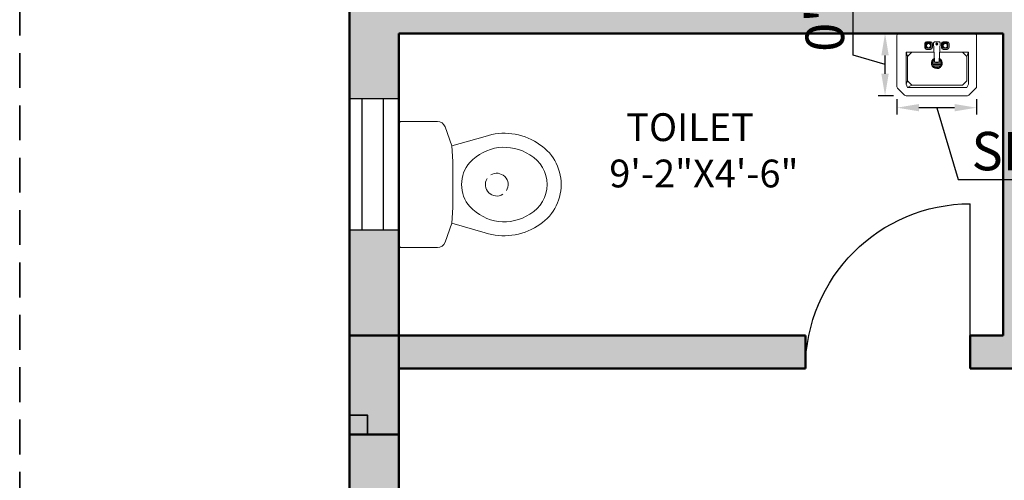
# Model space of a CAD drawing. Units: inches. Extents: x -7 to 1228, y -146 to 1091.
# Tile 5 of 88: x 0 to 179, y 193 to 276. Entities that reach past the tile are written whole.
import ezdxf

# ---------------------------------------------------------------- set-up
doc = ezdxf.new("R2010")
doc.units = ezdxf.units.IN
doc.linetypes.add('DASHED2', pattern=[9.525, 6.35, -3.175])
for name, color, linetype, lineweight in [('A-ANNO-DIMS', 2, 'Continuous', 18), ('A-AREA-IDEN', 7, 'Continuous', 18), ('A-COLS', 6, 'Continuous', 35), ('A-DOOR', 4, 'Continuous', 25), ('A-FLOR-FIXT', 8, 'Continuous', 18), ('A-FURN', 8, 'Continuous', 18), ('A-GLAZ', 175, 'Continuous', 25), ('A-WALL', 7, 'Continuous', 50), ('A-WALL-PATT', 251, 'Continuous', 13), ('C-PROP', 1, 'DASHED2', 35)]:
    doc.layers.add(name, color=color, linetype=linetype, lineweight=lineweight)
doc.styles.get("Standard").update_dxf_attribs({"font": 'arial.ttf'})
doc.dimstyles.new('ISO-25', dxfattribs={"dimtxt": 7, "dimasz": 4, "dimexe": 1.25, "dimexo": 0.625, "dimtad": 1, "dimdec": 1, "dimlunit": 3, "dimtxsty": 'Standard', "dimcen": 2.5, "dimadec": 0, "dimazin": 0, "dimtfac": 1, "dimtdec": 1, "dimtmove": 1, "dimatfit": 3, "dimfxl": 1, "dimarcsym": 0})

# ---------------------------------------------------------------- blocks, each defined once
blk = doc.blocks.new('A$C7B5C7CD4')
at = {"ltscale": 20}
for p, q in [((0, 0.614), (0, 0.4765)), ((0.243, 0.625), (0.011, 0.625)), ((0.243, 0.625), (0.475, 0.625)), ((0.486, 0.614), (0.486, 0.4765)), ((0.0212, 0.4467), (0.0946, 0.4214)), ((0.0946, 0.4214), (0.0576, 0.293)), ((0.0946, 0.4214), (0.1544, 0.4173)), ((0.3316, 0.4173), (0.1544, 0.4173)), ((0.3914, 0.4214), (0.3316, 0.4173)), ((0.4648, 0.4467), (0.3914, 0.4214)), ((0.3914, 0.4214), (0.4284, 0.293))]:
    blk.add_line(p, q, dxfattribs=at)
for centre, radius, start, end in [((0.011, 0.614), 0.011, 90, 180), ((0.475, 0.614), 0.011, 0, 90), ((0.0315, 0.4765), 0.0315, 180, 251), ((0.4545, 0.4765), 0.0315, 289, 0), ((0.24, 0.2602), 0.123, 88.6158, 131.7414), ((0.246, 0.2602), 0.123, 48.2586, 91.3842), ((0.2796, 0.219), 0.18, 132.4207, 213.289), ((0.2064, 0.219), 0.18, 326.711, 47.5793), ((0.2796, 0.219), 0.234, 161.5846, 212.8753), ((0.2064, 0.219), 0.234, 327.1247, 18.4154), ((0.243, 0.185), 0.131, 209.6292, 270), ((0.243, 0.185), 0.131, 270, 330.3708), ((0.243, 0.185), 0.185, 210.1745, 270), ((0.243, 0.185), 0.185, 270, 329.8255)]:
    blk.add_arc(centre, radius, start, end, dxfattribs=at)
for start, end in [(58.1785, 211.8215), (238.1785, 31.8215)]:
    blk.add_arc((0.2426, 0.2481), 0.0439, start, end)
blk = doc.blocks.new('A$C4CB854FF')
for p, q in [((0, 0.3675), (0, 0.0552)), ((0.4725, 0.38), (0.0125, 0.38)), ((0.485, 0.0552), (0.485, 0.3675)), ((0.1677, 0.2932), (0.1677, 0.318)), ((0.1745, 0.2919), (0.1745, 0.3194)), ((0.1773, 0.3221), (0.2048, 0.3221)), ((0.1787, 0.329), (0.2034, 0.329)), ((0.2075, 0.3194), (0.2075, 0.2919)), ((0.2144, 0.318), (0.2144, 0.2932)), ((0.2279, 0.2104), (0.2213, 0.3235)), ((0.2337, 0.329), (0.2502, 0.329)), ((0.2625, 0.3235), (0.256, 0.2104)), ((0.2694, 0.318), (0.2694, 0.2932)), ((0.2763, 0.3194), (0.2763, 0.2919)), ((0.3065, 0.3221), (0.279, 0.3221)), ((0.3052, 0.329), (0.2804, 0.329)), ((0.3093, 0.2919), (0.3093, 0.3194)), ((0.3162, 0.2932), (0.3162, 0.318)), ((0.05, 0.265), (0.2247, 0.265)), ((0.06, 0.24), (0.05, 0.265)), ((0.05, 0.07), (0.05, 0.265)), ((0.085, 0.265), (0.06, 0.24)), ((0.2048, 0.2891), (0.1773, 0.2891)), ((0.2034, 0.2822), (0.1787, 0.2822)), ((0.2591, 0.265), (0.43, 0.265)), ((0.279, 0.2891), (0.3065, 0.2891)), ((0.2804, 0.2822), (0.3052, 0.2822)), ((0.395, 0.265), (0.42, 0.24)), ((0.42, 0.24), (0.43, 0.265)), ((0.43, 0.07), (0.43, 0.265)), ((0.06, 0.24), (0.06, 0.09)), ((0.2152, 0.1984), (0.2694, 0.1984)), ((0.2297, 0.2066), (0.2165, 0.2066)), ((0.2681, 0.1901), (0.2165, 0.1901)), ((0.2272, 0.2149), (0.2208, 0.2149)), ((0.2638, 0.1819), (0.2208, 0.1819)), ((0.2505, 0.2052), (0.2334, 0.2052)), ((0.2681, 0.2066), (0.2541, 0.2066)), ((0.2638, 0.2149), (0.2566, 0.2149)), ((0.42, 0.24), (0.42, 0.09)), ((0.2533, 0.1736), (0.2313, 0.1736)), ((0.05, 0.07), (0.06, 0.05)), ((0.06, 0.09), (0.085, 0.065)), ((0.085, 0.065), (0.395, 0.065)), ((0.42, 0.09), (0.395, 0.065)), ((0.395, 0.065), (0.42, 0.05)), ((0.42, 0.09), (0.43, 0.07)), ((0.43, 0.07), (0.42, 0.05)), ((0.0037, 0.0463), (0.0463, 0.0037)), ((0.42, 0.05), (0.06, 0.05)), ((0.4387, 0.0037), (0.4813, 0.0463)), ((0.0552, 0), (0.4298, 0))]:
    blk.add_line(p, q)
for centre, radius in [((0.191, 0.3056), 0.0165), ((0.191, 0.3056), 0.0127), ((0.2419, 0.3152), 0.00688), ((0.2419, 0.3152), 0.00344), ((0.2928, 0.3056), 0.0165), ((0.2928, 0.3056), 0.0127)]:
    blk.add_circle(centre, radius)
for centre, radius, start, end in [((0.0125, 0.3675), 0.0125, 90, 180), ((0.4725, 0.3675), 0.0125, 0, 90), ((0.1787, 0.318), 0.011, 90, 180), ((0.1773, 0.3194), 0.00275, 90, 180), ((0.2034, 0.318), 0.011, 0, 90), ((0.2048, 0.3194), 0.00275, 360, 90), ((0.2329, 0.314), 0.015, 87.19754, 140.72744), ((0.2509, 0.314), 0.015, 39.27256, 92.80246), ((0.2804, 0.318), 0.011, 90, 180), ((0.279, 0.3194), 0.00275, 90, 180), ((0.3052, 0.318), 0.011, 0, 90), ((0.3065, 0.3194), 0.00275, 360, 90), ((0.1787, 0.2932), 0.011, 180, 270), ((0.1773, 0.2919), 0.00275, 180, 270), ((0.2034, 0.2932), 0.011, 270, 0), ((0.2048, 0.2919), 0.00275, 270, 0), ((0.2804, 0.2932), 0.011, 180, 270), ((0.279, 0.2919), 0.00275, 180, 270), ((0.3052, 0.2932), 0.011, 270, 360), ((0.3065, 0.2919), 0.00275, 270, 0), ((0.2423, 0.1984), 0.033, 118.68833, 62.86857), ((0.2423, 0.1984), 0.0271, 124.77581, 57.22467), ((0.2334, 0.2107), 0.0055, 183.3274, 270), ((0.2505, 0.2107), 0.0055, 270, 356.6726), ((0.0125, 0.0552), 0.0125, 180, 225), ((0.0552, 0.0125), 0.0125, 225, 270), ((0.4298, 0.0125), 0.0125, 270, 315), ((0.4725, 0.0552), 0.0125, 315, 0)]:
    blk.add_arc(centre, radius, start, end)
blk = doc.blocks.new('WIN-24')
for p, q in [((0, 0), (0, 24)), ((0, 24), (9, 24)), ((2.34, 0), (2.34, 24)), ((2.34, 24), (6.14, 24)), ((6.14, 24), (6.14, 0)), ((9, 24), (9, 0)), ((9, 0), (0, 0))]:
    blk.add_line(p, q)
blk = doc.blocks.new('DOOR-750')
blk.add_line((30, 30), (30, 0))
blk.add_arc((30, 30), 30, 180, 270)
blk = doc.blocks.new('*D32')
at = {"layer": 'A-ANNO-DIMS', "color": 0, "lineweight": -2, "transparency": 16777216}
for p, q in [((159.65, 262.03), (159.65, 259.24)), ((174.13, 262.03), (174.13, 259.24)), ((170.13, 260.49), (163.65, 260.49)), ((166.89, 260.49), (170.8, 247.44)), ((170.8, 247.44), (294.04, 247.44))]:
    blk.add_line(p, q, dxfattribs=at)
at = {"layer": 'A-ANNO-DIMS', "color": 0, "transparency": 16777216}
for points in [[(163.65, 261.15), (163.65, 259.82), (159.65, 260.49)], [(170.13, 261.15), (170.13, 259.82), (174.13, 260.49)]]:
    blk.add_solid(points, dxfattribs=at)
at = {"layer": 'Defpoints', "color": 0, "transparency": 16777216}
for p in [(159.65, 262.66), (174.13, 262.66), (159.65, 260.49)]:
    blk.add_point(p, dxfattribs=at)
at = {"layer": 'A-ANNO-DIMS', "color": 0, "transparency": 16777216, "insert": (232.42, 251.68), "char_height": 7, "attachment_point": 5}
blk.add_mtext('SINK / BASIN 1\'-2 1/2" TYP.', dxfattribs=at)
blk = doc.blocks.new('*D33')
at = {"layer": 'A-ANNO-DIMS', "color": 0, "lineweight": -2, "transparency": 16777216}
for p, q in [((151.67, 270.07), (151.67, 335.74)), ((159.03, 274), (156.23, 274)), ((157.48, 268.33), (151.67, 270.07)), ((157.48, 266.66), (157.48, 270)), ((159.03, 262.66), (156.23, 262.66))]:
    blk.add_line(p, q, dxfattribs=at)
at = {"layer": 'A-ANNO-DIMS', "color": 0, "transparency": 16777216}
for points in [[(156.81, 270), (158.15, 270), (157.48, 274)], [(156.81, 266.66), (158.15, 266.66), (157.48, 262.66)]]:
    blk.add_solid(points, dxfattribs=at)
at = {"layer": 'Defpoints', "color": 0, "transparency": 16777216}
for p in [(157.48, 274), (159.65, 274), (159.65, 262.66)]:
    blk.add_point(p, dxfattribs=at)
at = {"layer": 'A-ANNO-DIMS', "color": 0, "transparency": 16777216, "insert": (147.43, 302.9), "char_height": 7, "attachment_point": 5, "rotation": 90}
blk.add_mtext('0\'-11 1/2" TYP.', dxfattribs=at)

msp = doc.modelspace()

# ---------------------------------------------------------------- hatches: boundary and pattern name
at = {"layer": 'A-COLS'}
h = msp.add_hatch(color=256, dxfattribs=at)
h.dxf.hatch_style = 1
h.paths.add_polyline_path([(60, 204.55), (63.29, 204.55), (63.29, 201), (69, 201), (69, 219), (60, 219)])
h = msp.add_hatch(color=256, dxfattribs=at)
h.dxf.hatch_style = 1
h.paths.add_polyline_path([(60, 204.55), (60, 201), (63.29, 201), (63.29, 204.55)])
at = {"layer": 'A-WALL-PATT'}
h = msp.add_hatch(color=256, dxfattribs=at)
h.dxf.hatch_style = 1
h.paths.add_polyline_path([(69, 568), (60, 568), (60, 493), (63.29, 493), (69, 493)])
h.paths.add_polyline_path([(69, 662.41), (60, 662.41), (60, 586), (69, 586)], flags=17)
h.paths.add_polyline_path([(69, 723), (184, 723), (184, 734), (179, 734), (179, 728), (69, 728), (69, 741.62), (60, 741.62), (60, 698.41), (69, 698.41)], flags=17)
h.paths.add_polyline_path([(69, 782), (231, 782), (231, 728), (231, 723), (231, 586), (236, 586), (236, 787), (69, 787), (69, 800.13), (60, 800.13), (60, 765.62), (69, 765.62)])
h.paths.add_polyline_path([(184, 842), (189, 842), (189, 848), (173, 848), (173, 842), (179, 842), (179, 787), (184, 787)])
h.paths.add_polyline_path([(118.22, 69), (69, 69), (69, 60), (118.22, 60)])
h.paths.add_polyline_path([(227, 69), (154.22, 69), (154.22, 60), (227, 60)])
h.paths.add_polyline_path([(236, 60), (232.71, 60), (227, 60), (227, 36), (236, 36)])
h.paths.add_polyline_path([(389, 60), (380, 60), (380, 36), (389, 36)])
h.paths.add_polyline_path([(384, 181), (380, 181), (380, 115), (380, 78), (384, 78)])
h.paths.add_polyline_path([(380, 115), (334.55, 115), (334.55, 109), (380, 109)])
h.paths.add_polyline_path([(274.55, 115), (236, 115), (236, 201), (232.71, 201), (231, 201), (231, 78), (236, 78), (236, 109), (274.55, 109)])
h.paths.add_polyline_path([(69, 123), (60, 123), (60, 78), (69, 78)])
h.paths.add_polyline_path([(69, 201), (60, 201), (60, 159), (69, 159)])
h.paths.add_polyline_path([(143, 219), (69, 219), (69, 213), (143, 213)], flags=17)
h.paths.add_polyline_path([(189, 219), (184, 219), (184, 274), (231, 274), (231, 219), (236, 219), (236, 279), (184, 279), (184, 297), (179, 297), (179, 279), (69, 279), (69, 290.91), (60, 290.91), (60, 262.18), (69, 262.18), (69, 274), (179, 274), (179, 219), (173, 219), (173, 213), (189, 213)])
h.paths.add_polyline_path([(69, 238.18), (60, 238.18), (60, 219), (69, 219)], flags=17)
h.paths.add_polyline_path([(69, 333), (60, 333), (60, 314.91), (69, 314.91), (69, 316.96)])
h.paths.add_polyline_path([(190, 338), (184, 338), (69, 338), (69, 333), (179, 333), (179, 327), (184, 327), (184, 333.02), (190, 333.05)])
h.paths.add_polyline_path([(69, 386.81), (60, 386.81), (60, 351), (69, 351)])
h.paths.add_polyline_path([(69, 475), (60, 475), (60, 422.81), (69, 422.81)])
h.paths.add_polyline_path([(236, 475), (231, 475), (231, 351.24), (236, 351.24)])
h.paths.add_polyline_path([(384, 475), (380, 475), (380, 362), (384, 362)])
h.paths.add_polyline_path([(547, 307), (439, 307), (439, 356), (445, 356), (445, 362), (433, 362), (433, 307), (380, 307), (380, 244), (380, 241), (384, 241), (384, 301), (433, 301), (433, 277), (439, 277), (439, 301), (547, 301)])
h.paths.add_polyline_path([(547, 241), (439, 241), (439, 247), (433, 247), (433, 235), (547, 235)])
h.paths.add_polyline_path([(450, 69), (440.29, 69), (424.89, 69), (389, 69), (389, 60), (450, 60)])
h.paths.add_polyline_path([(547, 69), (486, 69), (486, 60), (547, 60)])
h.paths.add_polyline_path([(556, 148.27), (547, 148.27), (547, 78), (556, 78)])
h.paths.add_polyline_path([(556, 223), (547, 223), (547, 195), (547, 184.27), (556, 184.27)])
h.paths.add_polyline_path([(556, 311.19), (547, 311.19), (547, 273.08), (556, 273.08)])
h.paths.add_polyline_path([(556, 344), (552.71, 344), (547, 344), (547, 335.19), (556, 335.19)])
h.paths.add_polyline_path([(556, 249.08), (547, 249.08), (547, 241), (556, 241)])
h.paths.add_polyline_path([(547, 362), (475, 362), (475, 356), (547, 356)], flags=0)
h.paths.add_polyline_path([(556, 399.62), (547, 399.62), (547, 362), (556, 362)])
h.paths.add_polyline_path([(556, 475), (547, 475), (547, 435.62), (556, 435.62)])
h.paths.add_polyline_path([(547, 493), (389, 493), (389, 487), (547, 487)])
h.paths.add_polyline_path([(380, 493), (278, 493), (278, 487), (380, 487)])
h.paths.add_polyline_path([(227, 493), (69, 493), (69, 487), (227, 487)])
h.paths.add_polyline_path([(643, 122.44), (634, 122.44), (634, 78), (643, 78)])
h.paths.add_polyline_path([(702.5, 69), (692.79, 69), (677.39, 69), (643, 69), (643, 60), (702.5, 60)])
h.paths.add_polyline_path([(798, 69), (738.5, 69), (738.5, 60), (798, 60)])
h.paths.add_polyline_path([(807, 60), (803.71, 60), (798, 60), (798, 36), (807, 36)])
h.paths.add_polyline_path([(807, 109), (846.75, 109), (846.75, 115), (807, 115), (807, 159), (802, 159), (802, 78), (807, 78)])
h.paths.add_polyline_path([(807, 201), (802, 201), (802, 195), (807, 195)])
h.paths.add_polyline_path([(643, 201), (634, 201), (634, 158.44), (643, 158.44)])
h.paths.add_polyline_path([(756, 225), (751, 225), (751, 219), (643, 219), (643, 213), (756, 213)])
h.paths.add_polyline_path([(643, 240.85), (634, 240.85), (634, 219), (643, 219)])
h.paths.add_polyline_path([(643, 274), (643, 288.63), (634, 288.63), (634, 264.85), (643, 264.85)])
h.paths.add_polyline_path([(802, 279), (756, 279), (756, 297), (751, 297), (751, 279), (643, 279), (643, 274), (751, 274), (751, 255), (756, 255), (756, 274), (802, 274)])
h.paths.add_polyline_path([(807, 333), (803.71, 333), (802, 333), (802, 279), (802, 274), (802, 219), (807, 219)])
h.paths.add_polyline_path([(956, 182), (951, 182), (951, 115), (906.75, 115), (906.75, 109), (951, 109), (951, 78), (956, 78)])
h.paths.add_polyline_path([(960, 60), (951, 60), (951, 36), (960, 36)])
h.paths.add_polyline_path([(1021, 69), (1005.78, 69), (960, 69), (960, 60), (1021, 60)])
h.paths.add_polyline_path([(956, 224), (951, 224), (951, 218), (956, 218)])
h.paths.add_polyline_path([(956, 302), (1004, 302), (1004, 278), (1010, 278), (1010, 302), (1118, 302), (1118, 290.81), (1127, 290.81), (1127, 326.97), (1118, 326.97), (1118, 320.97), (1118, 307), (1010, 307), (1010, 356), (1016, 356), (1016, 362), (1004, 362), (1004, 307), (951, 307), (951, 244), (951, 242), (954.29, 242), (956, 242)])
h.paths.add_polyline_path([(643, 333), (634, 333), (634, 312.63), (643, 312.63), (643, 316.96)])
h.paths.add_polyline_path([(756, 338), (643, 338), (643, 333), (751, 333), (751, 327), (756, 327)])
h.paths.add_polyline_path([(643, 388), (634, 388), (634, 351), (643, 351)])
h.paths.add_polyline_path([(807, 357), (802, 357), (802, 351), (807, 351)])
h.paths.add_polyline_path([(807, 475), (802, 475), (802, 393), (807, 393)])
h.paths.add_polyline_path([(643, 475), (634, 475), (634, 424), (643, 424)])
h.paths.add_polyline_path([(798, 493), (643, 493), (643, 487), (798, 487)])
h.paths.add_polyline_path([(634, 493), (556, 493), (556, 487), (634, 487)])
h.paths.add_polyline_path([(813, 493), (807, 493), (807, 487), (813, 487)])
h.paths.add_polyline_path([(951, 493), (849, 493), (849, 487), (951, 487)])
h.paths.add_polyline_path([(956, 484), (951, 484), (951, 374), (956, 374)])
h.paths.add_polyline_path([(1109, 493), (969, 493), (969, 487), (1109, 487)])
h.paths.add_polyline_path([(1127, 484), (1118, 484), (1118, 450.64), (1127, 450.64)])
h.paths.add_polyline_path([(1127, 414.64), (1118, 414.64), (1118, 365), (1127, 365)])
h.paths.add_polyline_path([(1109, 362), (1046, 362), (1046, 356), (1109, 356)], flags=17)
h.paths.add_polyline_path([(1127, 356), (1123.45, 356), (1118, 356), (1118, 350.97), (1127, 350.97)], flags=0)
h.paths.add_polyline_path([(1127, 266.81), (1118, 266.81), (1118, 262.36), (1118, 242), (1127, 242)], flags=17)
h.paths.add_polyline_path([(1118, 242), (1010, 242), (1010, 248), (1004, 248), (1004, 237), (1118, 237)])
h.paths.add_polyline_path([(1127, 224), (1118, 224), (1118, 170), (1127, 170)])
h.paths.add_polyline_path([(1127, 134), (1118, 134), (1118, 78), (1127, 78)])
h.paths.add_polyline_path([(1118, 69), (1057, 69), (1057, 60), (1118, 60)])
h.paths.add_polyline_path([(227, 571.55), (227, 574), (69, 574), (69, 568), (227, 568)])
h.paths.add_polyline_path([(380, 571.55), (380, 574), (278, 574), (278, 568), (380, 568)])
h.paths.add_polyline_path([(242, 574), (236, 574), (236, 568), (242, 568)])
h.paths.add_polyline_path([(547, 571.55), (547, 574), (389, 574), (389, 568), (547, 568)])
h.paths.add_polyline_path([(384, 733), (380, 733), (380, 586), (384, 586)])
h.paths.add_polyline_path([(556, 646), (634, 646), (634, 655), (547, 655), (547, 586), (556, 586)])
h.paths.add_polyline_path([(634, 574), (556, 574), (556, 568), (634, 568)])
h.paths.add_polyline_path([(643, 655), (634, 655), (634, 586), (643, 586)])
h.paths.add_polyline_path([(798, 574), (643, 574), (643, 568), (798, 568)])
h.paths.add_polyline_path([(643, 663.85), (634, 663.85), (634, 655), (643, 655)])
h.paths.add_polyline_path([(556, 676.97), (547, 676.97), (547, 655), (556, 655)])
h.paths.add_polyline_path([(556, 733), (547, 733), (547, 712.97), (556, 712.97)])
h.paths.add_polyline_path([(643, 710), (634, 710), (634, 699.85), (643, 699.85)])
h.paths.add_polyline_path([(807, 668), (802, 668), (802, 586), (807, 586)])
h.paths.add_polyline_path([(951, 574), (849, 574), (849, 568), (951, 568)])
h.paths.add_polyline_path([(956, 691), (951, 691), (951, 577), (956, 577)])
h.paths.add_polyline_path([(1109, 574), (969, 574), (969, 568), (1109, 568)])
h.paths.add_polyline_path([(1127, 643.4), (1118, 643.4), (1118, 577), (1127, 577)])
h.paths.add_polyline_path([(1127, 568), (1123.45, 568), (1118, 568), (1118, 493), (1127, 493)])
h.paths.add_polyline_path([(1127, 733), (1118, 733), (1118, 679.4), (1127, 679.4)])
h.paths.add_polyline_path([(1127, 777.35), (1118, 777.35), (1118, 770.04), (1118, 751), (1127, 751)], flags=17)
h.paths.add_polyline_path([(1118, 751), (1010, 751), (1010, 757), (1004, 757), (1004, 745), (1118, 745)])
h.paths.add_polyline_path([(956, 811), (1004, 811), (1004, 787), (1010, 787), (1010, 811), (1017.87, 811), (1017.87, 811.63, -0.414214), (1018.25, 812), (1031.98, 812, -0.414214), (1032.35, 811.63), (1032.35, 811), (1118, 811), (1118, 801.35), (1127, 801.35), (1127, 834.69), (1118, 834.69), (1118, 830.24), (1118, 817), (1010, 817), (1010, 866), (1016, 866), (1016, 872), (1004, 872), (1004, 817), (956, 817), (956, 866), (951, 866), (951, 751), (954.29, 751), (956, 751)])
h.paths.add_polyline_path([(1118, 872), (1046, 872), (1046, 866), (1118, 866)], flags=17)
h.paths.add_polyline_path([(1127, 924.71), (1118, 924.71), (1118, 884), (1127, 884)])
h.paths.add_polyline_path([(1127, 866), (1123.71, 866), (1118, 866), (1118, 858.69), (1127, 858.69)], flags=17)
h.paths.add_polyline_path([(956, 983), (951, 983), (951, 952), (807, 952), (807, 983), (802, 983), (802, 902), (807, 902), (807, 946), (951, 946), (951, 884), (956, 884)])
h.paths.add_polyline_path([(807, 842), (802, 842), (802, 787), (756, 787), (756, 806), (751, 806), (751, 787), (643, 787), (643, 782), (751, 782), (751, 764), (756, 764), (756, 782), (802, 782), (802, 728), (807, 728)])
h.paths.add_polyline_path([(756, 848), (643, 848), (643, 842), (751, 842), (751, 836), (756, 836)])
h.paths.add_polyline_path([(756, 734), (751, 734), (751, 728), (643, 728), (643, 723), (756, 723)])
h.paths.add_polyline_path([(643, 749.79), (634, 749.79), (634, 728), (637.29, 728), (643, 728)])
h.paths.add_polyline_path([(643, 805.41), (634, 805.41), (634, 773.79), (643, 773.79)])
h.paths.add_polyline_path([(643, 896.66), (634, 896.66), (634, 860), (637.29, 860), (643, 860)])
h.paths.add_polyline_path([(643, 842), (634, 842), (634, 829.41), (643, 829.41)])
h.paths.add_polyline_path([(643, 983), (634, 983), (634, 932.66), (643, 932.66)])
h.paths.add_polyline_path([(1127, 983), (1118, 983), (1118, 960.71), (1127, 960.71)])
h.paths.add_polyline_path([(1118, 1001), (1077.53, 1001), (1077.53, 992), (1118, 992)])
h.paths.add_polyline_path([(1041.53, 1001), (960, 1001), (960, 992), (1041.53, 992)])
h.paths.add_polyline_path([(960, 1025), (951, 1025), (951, 1001), (954.29, 1001), (960, 1001)])
h.paths.add_polyline_path([(807, 1025), (798, 1025), (798, 1001), (807, 1001)])
h.paths.add_polyline_path([(798, 1001), (738.5, 1001), (738.5, 992), (798, 992)])
h.paths.add_polyline_path([(702.5, 1001), (643, 1001), (643, 992), (702.5, 992)])
h.paths.add_polyline_path([(547, 1001), (499.11, 1001), (499.11, 992), (547, 992)])
h.paths.add_polyline_path([(463.11, 1001), (389, 1001), (389, 992), (463.11, 992)])
h.paths.add_polyline_path([(389, 1025), (380, 1025), (380, 1022), (380, 1001), (383.29, 1001), (389, 1001)])
h.paths.add_polyline_path([(236, 1025), (227, 1025), (227, 1001), (236, 1001)])
h.paths.add_polyline_path([(236, 983), (231, 983), (231, 860), (236, 860)])
h.paths.add_polyline_path([(274.55, 952), (236, 952), (236, 946), (274.55, 946)])
h.paths.add_polyline_path([(380, 952), (334.55, 952), (334.55, 946), (380, 946)])
h.paths.add_polyline_path([(384, 983), (380, 983), (380, 884), (383.29, 884), (384, 884)])
h.paths.add_polyline_path([(227, 1001), (155.01, 1001), (155.01, 992), (162.87, 992), (227, 992)])
h.paths.add_polyline_path([(119.01, 1001), (69, 1001), (69, 992), (119.01, 992)])
h.paths.add_polyline_path([(69, 983), (60, 983), (60, 922.99), (69, 922.99)])
h.paths.add_polyline_path([(69, 886.99), (60, 886.99), (60, 860), (63.29, 860), (69, 860)])
h.paths.add_polyline_path([(143, 848), (69, 848), (69, 842), (143, 842)])

# ---------------------------------------------------------------- linework, layer by layer
at = {"layer": 'A-COLS'}
msp.add_lwpolyline([(60, 201), (63.29, 201), (63.29, 204.55), (60, 204.55)], close=True, dxfattribs=at)
at = {"layer": 'A-WALL'}
for p, q in [((60, 1001), (60, 60)), ((69, 219), (69, 274)), ((179, 274), (69, 274)), ((69, 274), (69, 60)), ((179, 219), (179, 274)), ((69, 219), (60, 219)), ((60, 219), (60, 201)), ((143, 219), (69, 219)), ((69, 201), (69, 219)), ((143, 213), (143, 219)), ((179, 219), (173, 219)), ((173, 219), (173, 213)), ((143, 213), (69, 213)), ((69, 69), (69, 213)), ((189, 213), (173, 213)), ((60, 201), (69, 201))]:
    msp.add_line(p, q, dxfattribs=at)
at = {"layer": 'C-PROP'}
msp.add_line((0, 1061), (0, 0), dxfattribs=at)

# ---------------------------------------------------------------- block references
at = {"layer": 'A-DOOR', "extrusion": (0, 0, -1), "zscale": -1, "rotation": 180}
msp.add_blockref('DOOR-750', (-143, 243), dxfattribs=at)
at = {"layer": 'A-FLOR-FIXT', "xscale": 47.26153857112405, "yscale": 47.26153857112405, "zscale": 47.26153857112405, "rotation": 90}
msp.add_blockref('A$C7B5C7CD4', (98.54, 235.02), dxfattribs=at)
at = {"layer": 'A-FURN', "xscale": -29.84864686937646, "yscale": 29.84864686937646, "zscale": 29.84864686937646}
msp.add_blockref('A$C4CB854FF', (174.13, 262.66), dxfattribs=at)
at = {"layer": 'A-GLAZ'}
msp.add_blockref('WIN-24', (60, 238.18), dxfattribs=at)

# ---------------------------------------------------------------- texts
at = {"layer": 'A-AREA-IDEN', "insert": (107.3, 259.47), "char_height": 5.0568, "attachment_point": 1}
msp.add_mtext_dynamic_manual_height_columns('  TOILET\\P9\'-2"X4\'-6"', width=137.2821, gutter_width=25.28, heights=[0], dxfattribs=at)

# ---------------------------------------------------------------- dimensions: what is measured, and where the dimension line sits
at = {"layer": 'A-ANNO-DIMS'}
for base, p1, p2, angle, text, picture, middle in [((157.48, 274), (159.65, 262.66), (159.65, 274), 90, '<> TYP.', '*D33', (147.43, 270.7)), ((159.65, 260.49), (174.13, 262.66), (159.65, 262.66), 180, 'SINK / BASIN <> TYP.', '*D32', (171.43, 251.68))]:
    dim = msp.add_linear_dim(base=base, p1=p1, p2=p2, angle=angle, text=text, dimstyle='ISO-25', override={"dimdec": 1, "dimlfac": 1, "dimrnd": 0, "dimzin": 1, "dimdsep": 46, "dimlunit": 4, "dimfrac": 2}, dxfattribs=at)
    dim.commit()
    dim.dimension.update_dxf_attribs({"geometry": picture, "text_midpoint": middle})

doc.saveas('drawing.dxf')
